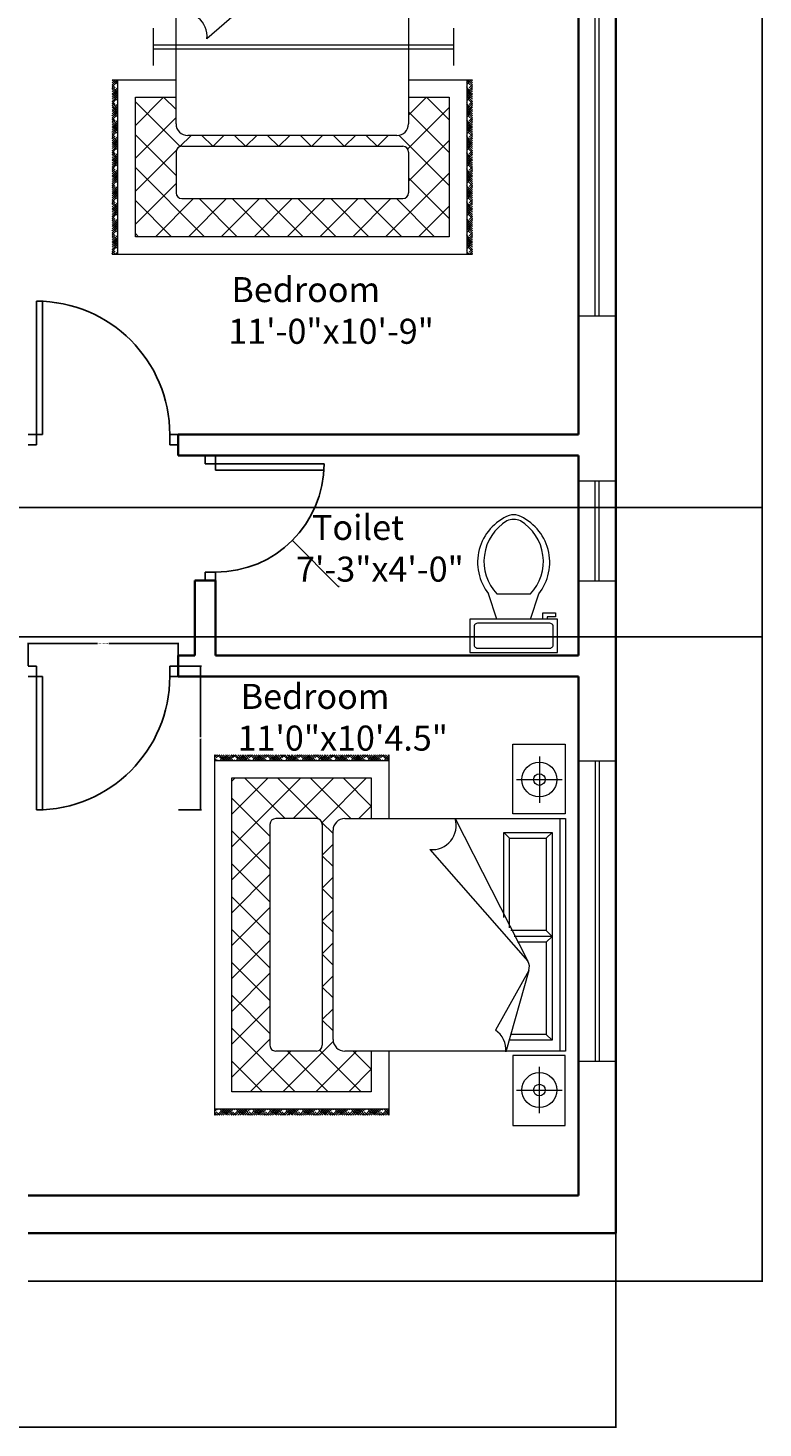
# Model space of a CAD drawing. Units: inches. Extents: x 3198 to 3702, y 1509 to 2253.
# Tile 3 of 6: x 3526 to 3702, y 1509 to 1845. Entities that reach past the tile are written whole.
import ezdxf

# ---------------------------------------------------------------- set-up
doc = ezdxf.new("R2010")
doc.units = ezdxf.units.IN
for name, color, linetype, lineweight in [('A-ANNO-DIMS', 2, 'Continuous', 18), ('A-AREA-IDEN', 7, 'Continuous', 18), ('A-DOOR', 3, 'Continuous', 25), ('A-FLOR-FIXT', 9, 'Continuous', 18), ('A-FURN', 8, 'Continuous', 13), ('A-GLAZ', 4, 'Continuous', 18), ('A-WALL', 7, 'Continuous', 35)]:
    doc.layers.add(name, color=color, linetype=linetype, lineweight=lineweight)
doc.styles.get("Standard").update_dxf_attribs({"font": 'arial.ttf'})
doc.dimstyles.get("Standard").update_dxf_attribs({"dimtxt": 0.18, "dimasz": 0.18, "dimexe": 0.18, "dimexo": 0.0625, "dimgap": 0.09, "dimtad": 0, "dimtih": 1, "dimtoh": 1, "dimdec": 4, "dimzin": 0, "dimdsep": 46, "dimtxsty": 'Standard', "dimcen": 0.09, "dimadec": 0, "dimazin": 0, "dimtfac": 1, "dimtdec": 4, "dimtofl": 0, "dimtmove": 0, "dimatfit": 3, "dimfxl": 1, "dimtolj": 1, "dimtzin": 0, "dimarcsym": 0})

# ---------------------------------------------------------------- blocks, each defined once
blk = doc.blocks.new('A$C4CB008C5')
for p, q in [((0, 3.019), (0.6, 3.019)), ((0, 2.569), (0, 3.019)), ((0.6, 3.019), (0.6, 2.569)), ((0.64, 1.121), (0.64, 3.021)), ((0.64, 3.021), (2.64, 3.021)), ((2.64, 3.021), (2.64, 1.121)), ((3.279, 3.019), (2.679, 3.019)), ((2.679, 3.019), (2.679, 2.569)), ((3.279, 2.569), (3.279, 3.019)), ((0.304, 2.6), (0.304, 2.992)), ((0.64, 2.971), (2.64, 2.971)), ((0.759, 2.905), (2.547, 2.905)), ((0.759, 2.489), (0.759, 2.905)), ((0.759, 2.905), (0.809, 2.855)), ((1.603, 2.855), (1.653, 2.905)), ((1.653, 2.905), (1.653, 2.579)), ((1.653, 2.905), (1.703, 2.855)), ((2.497, 2.855), (2.547, 2.905)), ((2.547, 2.905), (2.547, 2.54)), ((2.975, 2.6), (2.975, 2.992)), ((0.106, 2.796), (0.503, 2.796)), ((0.809, 2.855), (1.603, 2.855)), ((0.809, 2.539), (0.809, 2.855)), ((1.603, 2.855), (1.603, 2.551)), ((1.703, 2.855), (1.703, 2.607)), ((1.703, 2.855), (2.497, 2.855)), ((2.497, 2.855), (2.497, 2.556)), ((3.174, 2.796), (2.776, 2.796)), ((0.64, 2.071), (1.866, 2.698)), ((0.906, 1.854), (1.866, 2.698)), ((1.946, 2.705), (2.646, 2.507)), ((1.946, 2.705), (2.46, 2.418)), ((0.6, 2.569), (0, 2.569)), ((0.809, 2.539), (0.759, 2.489)), ((1.58, 2.539), (0.809, 2.539)), ((2.679, 2.569), (3.279, 2.569)), ((1.49, 2.489), (0.759, 2.489)), ((0.907, 1.867), (0.919, 1.867)), ((0.09, 1.5), (0.64, 1.5)), ((0.09, 1.491), (0.099, 1.5)), ((0.09, 1.473), (0.116, 1.5)), ((0.09, 1.456), (0.134, 1.5)), ((0.09, 1.474), (0.09, 1.475)), ((0.09, 1.438), (0.126, 1.474)), ((0.117, 1.43), (0.09, 1.457)), ((0.14, 1.46), (0.108, 1.492)), ((0.14, 1.478), (0.118, 1.5)), ((0.14, 1.496), (0.135, 1.5)), ((0.14, 1.442), (0.135, 1.448)), ((0.14, 0), (0.14, 1.5)), ((2.64, 1.5), (3.19, 1.5)), ((3.14, 1.496), (3.144, 1.5)), ((3.14, 1.478), (3.162, 1.5)), ((3.14, 1.5), (3.14, 0)), ((3.14, 1.46), (3.171, 1.492)), ((3.14, 1.442), (3.145, 1.448)), ((3.19, 1.456), (3.145, 1.5)), ((3.19, 1.438), (3.154, 1.474)), ((3.162, 1.43), (3.19, 1.457)), ((3.19, 1.473), (3.163, 1.5)), ((3.19, 1.491), (3.181, 1.5)), ((3.189, 1.474), (3.19, 1.475)), ((0.14, 1.389), (0.09, 1.439)), ((0.09, 1.42), (0.099, 1.43)), ((0.14, 1.372), (0.09, 1.422)), ((0.09, 1.368), (0.14, 1.417)), ((0.14, 1.354), (0.09, 1.404)), ((0.09, 1.35), (0.14, 1.4)), ((0.14, 1.336), (0.09, 1.386)), ((0.09, 1.332), (0.14, 1.382)), ((0.09, 1.314), (0.14, 1.364)), ((0.09, 1.297), (0.126, 1.333)), ((0.09, 1.333), (0.09, 1.333)), ((0.14, 1.319), (0.108, 1.35)), ((0.117, 1.412), (0.14, 1.435)), ((0.29, 1.108), (0.532, 1.35)), ((0.29, 0.15), (0.29, 1.35)), ((0.29, 1.35), (0.64, 1.35)), ((0.64, 1.243), (0.533, 1.35)), ((2.64, 1.195), (2.795, 1.35)), ((2.64, 1.35), (2.99, 1.35)), ((2.99, 1.156), (2.795, 1.35)), ((2.99, 1.35), (2.99, 0.15)), ((3.14, 1.389), (3.19, 1.439)), ((3.162, 1.412), (3.14, 1.435)), ((3.14, 1.372), (3.19, 1.422)), ((3.189, 1.368), (3.14, 1.417)), ((3.14, 1.354), (3.19, 1.404)), ((3.19, 1.35), (3.14, 1.4)), ((3.14, 1.336), (3.19, 1.386)), ((3.19, 1.332), (3.14, 1.382)), ((3.19, 1.314), (3.14, 1.364)), ((3.14, 1.319), (3.171, 1.35)), ((3.19, 1.297), (3.154, 1.333)), ((3.19, 1.42), (3.18, 1.43)), ((3.189, 1.333), (3.19, 1.333)), ((0.117, 1.288), (0.09, 1.316)), ((0.14, 1.248), (0.09, 1.298)), ((0.09, 1.279), (0.099, 1.288)), ((0.14, 1.23), (0.09, 1.28)), ((0.09, 1.227), (0.14, 1.276)), ((0.14, 1.213), (0.09, 1.263)), ((0.09, 1.208), (0.14, 1.258)), ((0.14, 1.195), (0.09, 1.245)), ((0.09, 1.19), (0.14, 1.24)), ((0.09, 1.173), (0.14, 1.223)), ((0.14, 1.177), (0.108, 1.209)), ((0.117, 1.271), (0.14, 1.294)), ((0.14, 1.301), (0.135, 1.306)), ((0.674, 0.926), (0.29, 1.31)), ((2.632, 0.904), (2.99, 1.262)), ((2.99, 0.873), (2.64, 1.223)), ((3.14, 1.301), (3.145, 1.306)), ((3.14, 1.248), (3.19, 1.298)), ((3.162, 1.271), (3.14, 1.294)), ((3.14, 1.23), (3.19, 1.28)), ((3.189, 1.227), (3.14, 1.276)), ((3.14, 1.213), (3.19, 1.263)), ((3.19, 1.208), (3.14, 1.258)), ((3.14, 1.195), (3.19, 1.245)), ((3.19, 1.19), (3.14, 1.24)), ((3.19, 1.173), (3.14, 1.223)), ((3.14, 1.177), (3.171, 1.209)), ((3.162, 1.288), (3.19, 1.316)), ((3.19, 1.279), (3.18, 1.288)), ((0.09, 1.191), (0.09, 1.192)), ((0.09, 1.155), (0.126, 1.191)), ((0.117, 1.147), (0.09, 1.174)), ((0.14, 1.107), (0.09, 1.157)), ((0.09, 1.137), (0.099, 1.147)), ((0.14, 1.089), (0.09, 1.139)), ((0.09, 1.085), (0.14, 1.134)), ((0.14, 1.071), (0.09, 1.121)), ((0.09, 1.067), (0.14, 1.117)), ((0.14, 1.054), (0.09, 1.104)), ((0.09, 1.049), (0.14, 1.099)), ((0.117, 1.129), (0.14, 1.152)), ((0.14, 1.16), (0.135, 1.165)), ((0.29, 0.825), (0.64, 1.175)), ((3.14, 1.16), (3.145, 1.165)), ((3.14, 1.107), (3.19, 1.157)), ((3.162, 1.129), (3.14, 1.152)), ((3.14, 1.089), (3.19, 1.139)), ((3.189, 1.085), (3.14, 1.134)), ((3.14, 1.071), (3.19, 1.121)), ((3.19, 1.067), (3.14, 1.117)), ((3.14, 1.054), (3.19, 1.104)), ((3.19, 1.049), (3.14, 1.099)), ((3.19, 1.155), (3.154, 1.191)), ((3.162, 1.147), (3.19, 1.174)), ((3.19, 1.137), (3.18, 1.147)), ((3.189, 1.191), (3.19, 1.192)), ((0.09, 1.031), (0.14, 1.081)), ((0.09, 1.05), (0.09, 1.051)), ((0.09, 1.014), (0.126, 1.05)), ((0.117, 1.006), (0.09, 1.033)), ((0.14, 0.965), (0.09, 1.015)), ((0.09, 0.996), (0.099, 1.006)), ((0.14, 0.948), (0.09, 0.998)), ((0.09, 0.944), (0.14, 0.993)), ((0.14, 0.93), (0.09, 0.98)), ((0.09, 0.925), (0.14, 0.975)), ((0.14, 1.036), (0.108, 1.067)), ((0.117, 0.988), (0.14, 1.011)), ((0.14, 1.018), (0.135, 1.023)), ((0.64, 0.677), (0.29, 1.027)), ((0.673, 0.925), (0.769, 1.021)), ((2.54, 1.021), (0.74, 1.021)), ((0.955, 0.928), (0.861, 1.021)), ((0.959, 0.928), (1.052, 1.021)), ((1.238, 0.928), (1.144, 1.021)), ((1.241, 0.928), (1.335, 1.021)), ((1.52, 0.928), (1.427, 1.021)), ((1.524, 0.928), (1.618, 1.021)), ((1.803, 0.928), (1.71, 1.021)), ((1.807, 0.928), (1.9, 1.021)), ((2.086, 0.928), (1.993, 1.021)), ((2.09, 0.928), (2.183, 1.021)), ((2.369, 0.928), (2.276, 1.021)), ((2.373, 0.928), (2.466, 1.021)), ((2.99, 0.59), (2.557, 1.023)), ((2.64, 0.629), (2.99, 0.979)), ((3.19, 1.031), (3.14, 1.081)), ((3.14, 1.036), (3.171, 1.067)), ((3.14, 1.018), (3.145, 1.023)), ((3.14, 0.965), (3.19, 1.015)), ((3.162, 0.988), (3.14, 1.011)), ((3.14, 0.948), (3.19, 0.998)), ((3.189, 0.944), (3.14, 0.993)), ((3.14, 0.93), (3.19, 0.98)), ((3.19, 0.925), (3.14, 0.975)), ((3.19, 1.014), (3.154, 1.05)), ((3.162, 1.006), (3.19, 1.033)), ((3.19, 0.996), (3.18, 1.006)), ((3.189, 1.05), (3.19, 1.051)), ((0.14, 0.912), (0.09, 0.962)), ((0.09, 0.908), (0.14, 0.958)), ((0.09, 0.89), (0.14, 0.94)), ((0.09, 0.908), (0.09, 0.909)), ((0.09, 0.872), (0.126, 0.908)), ((0.117, 0.864), (0.09, 0.891)), ((0.14, 0.824), (0.09, 0.874)), ((0.09, 0.855), (0.099, 0.864)), ((0.14, 0.806), (0.09, 0.856)), ((0.09, 0.802), (0.14, 0.852)), ((0.14, 0.894), (0.108, 0.926)), ((0.117, 0.847), (0.14, 0.869)), ((0.14, 0.877), (0.135, 0.882)), ((0.29, 0.542), (0.643, 0.895)), ((0.64, 0.878), (0.64, 0.528)), ((0.69, 0.928), (2.59, 0.928)), ((2.64, 0.878), (2.64, 0.528)), ((3.14, 0.912), (3.19, 0.962)), ((3.19, 0.908), (3.14, 0.958)), ((3.19, 0.89), (3.14, 0.94)), ((3.14, 0.894), (3.171, 0.926)), ((3.14, 0.877), (3.145, 0.882)), ((3.14, 0.824), (3.19, 0.874)), ((3.162, 0.847), (3.14, 0.869)), ((3.14, 0.806), (3.19, 0.856)), ((3.189, 0.802), (3.14, 0.852)), ((3.19, 0.872), (3.154, 0.908)), ((3.162, 0.864), (3.19, 0.891)), ((3.19, 0.855), (3.18, 0.864)), ((3.189, 0.908), (3.19, 0.909)), ((0.14, 0.788), (0.09, 0.838)), ((0.09, 0.784), (0.14, 0.834)), ((0.14, 0.771), (0.09, 0.821)), ((0.09, 0.766), (0.14, 0.816)), ((0.09, 0.749), (0.14, 0.799)), ((0.09, 0.767), (0.09, 0.768)), ((0.09, 0.731), (0.126, 0.767)), ((0.117, 0.723), (0.09, 0.75)), ((0.14, 0.682), (0.09, 0.732)), ((0.09, 0.713), (0.099, 0.723)), ((0.14, 0.753), (0.108, 0.785)), ((0.117, 0.705), (0.14, 0.728)), ((0.14, 0.735), (0.135, 0.74)), ((0.884, 0.15), (0.29, 0.744)), ((3.14, 0.788), (3.19, 0.838)), ((3.19, 0.784), (3.14, 0.834)), ((3.14, 0.771), (3.19, 0.821)), ((3.19, 0.766), (3.14, 0.816)), ((3.19, 0.749), (3.14, 0.799)), ((3.14, 0.753), (3.171, 0.785)), ((3.14, 0.735), (3.145, 0.74)), ((3.14, 0.682), (3.19, 0.732)), ((3.162, 0.705), (3.14, 0.728)), ((3.19, 0.731), (3.154, 0.767)), ((3.162, 0.723), (3.19, 0.75)), ((3.19, 0.713), (3.18, 0.723)), ((3.189, 0.767), (3.19, 0.768)), ((0.14, 0.665), (0.09, 0.715)), ((0.09, 0.661), (0.14, 0.71)), ((0.14, 0.647), (0.09, 0.697)), ((0.09, 0.642), (0.14, 0.692)), ((0.14, 0.629), (0.09, 0.679)), ((0.09, 0.625), (0.14, 0.675)), ((0.09, 0.607), (0.14, 0.657)), ((0.09, 0.589), (0.126, 0.626)), ((0.09, 0.626), (0.09, 0.626)), ((0.117, 0.581), (0.09, 0.609)), ((0.14, 0.612), (0.108, 0.643)), ((0.29, 0.259), (0.64, 0.609)), ((2.443, 0.15), (2.99, 0.696)), ((2.99, 0.307), (2.64, 0.657)), ((3.14, 0.665), (3.19, 0.715)), ((3.189, 0.661), (3.14, 0.71)), ((3.14, 0.647), (3.19, 0.697)), ((3.19, 0.642), (3.14, 0.692)), ((3.14, 0.629), (3.19, 0.679)), ((3.19, 0.625), (3.14, 0.675)), ((3.19, 0.607), (3.14, 0.657)), ((3.14, 0.612), (3.171, 0.643)), ((3.19, 0.589), (3.154, 0.626)), ((3.162, 0.581), (3.19, 0.609)), ((3.189, 0.626), (3.19, 0.626)), ((0.14, 0.541), (0.09, 0.591)), ((0.09, 0.572), (0.099, 0.581)), ((0.14, 0.523), (0.09, 0.573)), ((0.09, 0.519), (0.14, 0.569)), ((0.14, 0.506), (0.09, 0.556)), ((0.09, 0.501), (0.14, 0.551)), ((0.14, 0.488), (0.09, 0.538)), ((0.09, 0.483), (0.14, 0.533)), ((0.09, 0.466), (0.14, 0.516)), ((0.09, 0.484), (0.09, 0.485)), ((0.09, 0.448), (0.126, 0.484)), ((0.14, 0.47), (0.108, 0.502)), ((0.117, 0.564), (0.14, 0.586)), ((0.14, 0.594), (0.135, 0.599)), ((3.14, 0.594), (3.145, 0.599)), ((3.14, 0.541), (3.19, 0.591)), ((3.162, 0.564), (3.14, 0.586)), ((3.14, 0.523), (3.19, 0.573)), ((3.189, 0.519), (3.14, 0.569)), ((3.14, 0.506), (3.19, 0.556)), ((3.19, 0.501), (3.14, 0.551)), ((3.14, 0.488), (3.19, 0.538)), ((3.19, 0.483), (3.14, 0.533)), ((3.19, 0.466), (3.14, 0.516)), ((3.14, 0.47), (3.171, 0.502)), ((3.19, 0.448), (3.154, 0.484)), ((3.19, 0.572), (3.18, 0.581)), ((3.189, 0.484), (3.19, 0.485)), ((0.117, 0.44), (0.09, 0.467)), ((0.14, 0.399), (0.09, 0.449)), ((0.09, 0.43), (0.099, 0.44)), ((0.14, 0.382), (0.09, 0.432)), ((0.09, 0.378), (0.14, 0.427)), ((0.14, 0.364), (0.09, 0.414)), ((0.09, 0.36), (0.14, 0.41)), ((0.14, 0.346), (0.09, 0.396)), ((0.09, 0.342), (0.14, 0.392)), ((0.09, 0.324), (0.14, 0.374)), ((0.117, 0.422), (0.14, 0.445)), ((0.14, 0.453), (0.135, 0.458)), ((0.601, 0.15), (0.29, 0.462)), ((0.463, 0.15), (0.791, 0.478)), ((0.69, 0.478), (2.59, 0.478)), ((0.746, 0.15), (1.074, 0.478)), ((1.167, 0.15), (0.839, 0.478)), ((1.029, 0.15), (1.357, 0.478)), ((1.45, 0.15), (1.122, 0.478)), ((1.312, 0.15), (1.64, 0.478)), ((1.733, 0.15), (1.405, 0.478)), ((1.595, 0.15), (1.923, 0.478)), ((2.016, 0.15), (1.688, 0.478)), ((1.878, 0.15), (2.206, 0.478)), ((2.298, 0.15), (1.97, 0.478)), ((2.16, 0.15), (2.488, 0.478)), ((2.581, 0.15), (2.253, 0.478)), ((2.864, 0.15), (2.536, 0.478)), ((2.726, 0.15), (2.99, 0.414)), ((3.14, 0.453), (3.145, 0.458)), ((3.14, 0.399), (3.19, 0.449)), ((3.162, 0.422), (3.14, 0.445)), ((3.14, 0.382), (3.19, 0.432)), ((3.189, 0.378), (3.14, 0.427)), ((3.14, 0.364), (3.19, 0.414)), ((3.19, 0.36), (3.14, 0.41)), ((3.14, 0.346), (3.19, 0.396)), ((3.19, 0.342), (3.14, 0.392)), ((3.19, 0.324), (3.14, 0.374)), ((3.162, 0.44), (3.19, 0.467)), ((3.19, 0.43), (3.18, 0.44)), ((0.09, 0.307), (0.126, 0.343)), ((0.09, 0.343), (0.09, 0.343)), ((0.117, 0.299), (0.09, 0.326)), ((0.14, 0.258), (0.09, 0.308)), ((0.09, 0.289), (0.099, 0.299)), ((0.14, 0.24), (0.09, 0.29)), ((0.09, 0.237), (0.14, 0.286)), ((0.14, 0.223), (0.09, 0.273)), ((0.09, 0.218), (0.14, 0.268)), ((0.14, 0.205), (0.09, 0.255)), ((0.09, 0.201), (0.14, 0.251)), ((0.14, 0.329), (0.108, 0.36)), ((0.117, 0.281), (0.14, 0.304)), ((0.14, 0.311), (0.135, 0.316)), ((3.14, 0.329), (3.171, 0.36)), ((3.14, 0.311), (3.145, 0.316)), ((3.14, 0.258), (3.19, 0.308)), ((3.162, 0.281), (3.14, 0.304)), ((3.14, 0.24), (3.19, 0.29)), ((3.189, 0.237), (3.14, 0.286)), ((3.14, 0.223), (3.19, 0.273)), ((3.19, 0.218), (3.14, 0.268)), ((3.14, 0.205), (3.19, 0.255)), ((3.19, 0.201), (3.14, 0.251)), ((3.19, 0.307), (3.154, 0.343)), ((3.162, 0.299), (3.19, 0.326)), ((3.19, 0.289), (3.18, 0.299)), ((3.189, 0.343), (3.19, 0.343)), ((0.09, 0.183), (0.14, 0.233)), ((0.09, 0.201), (0.09, 0.202)), ((0.09, 0.165), (0.126, 0.201)), ((0.117, 0.157), (0.09, 0.184)), ((0.14, 0.117), (0.09, 0.167)), ((0.09, 0.148), (0.099, 0.157)), ((0.14, 0.099), (0.09, 0.149)), ((0.09, 0.095), (0.14, 0.144)), ((0.14, 0.081), (0.09, 0.131)), ((0.09, 0.077), (0.14, 0.127)), ((0.14, 0.187), (0.108, 0.219)), ((0.117, 0.139), (0.14, 0.162)), ((0.14, 0.17), (0.135, 0.175)), ((0.318, 0.15), (0.29, 0.179)), ((2.99, 0.15), (0.29, 0.15)), ((3.19, 0.183), (3.14, 0.233)), ((3.14, 0.187), (3.171, 0.219)), ((3.14, 0.17), (3.145, 0.175)), ((3.14, 0.117), (3.19, 0.167)), ((3.162, 0.139), (3.14, 0.162)), ((3.14, 0.099), (3.19, 0.149)), ((3.189, 0.095), (3.14, 0.144)), ((3.14, 0.081), (3.19, 0.131)), ((3.19, 0.077), (3.14, 0.127)), ((3.19, 0.165), (3.154, 0.201)), ((3.162, 0.157), (3.19, 0.184)), ((3.19, 0.148), (3.18, 0.157)), ((3.189, 0.201), (3.19, 0.202)), ((0.14, 0.064), (0.09, 0.114)), ((0.09, 0.059), (0.14, 0.109)), ((0.09, 0.041), (0.14, 0.091)), ((0.09, 0.06), (0.09, 0.061)), ((0.09, 0.024), (0.126, 0.06)), ((0.117, 0.016), (0.09, 0.043)), ((0.115, 0), (0.09, 0.025)), ((0.09, 0.006), (0.099, 0.016)), ((0.097, 0), (0.09, 0.008)), ((0.14, 0.046), (0.108, 0.078)), ((0.119, 0), (0.14, 0.021)), ((0.14, 0.028), (0.135, 0.033)), ((0.137, 0), (0.14, 0.003)), ((3.14, 0.064), (3.19, 0.114)), ((3.19, 0.059), (3.14, 0.109)), ((3.19, 0.041), (3.14, 0.091)), ((3.14, 0.046), (3.171, 0.078)), ((3.14, 0.028), (3.145, 0.033)), ((3.16, 0), (3.14, 0.021)), ((3.143, 0), (3.14, 0.003)), ((3.19, 0.024), (3.154, 0.06)), ((3.162, 0.016), (3.19, 0.043)), ((3.164, 0), (3.19, 0.025)), ((3.19, 0.006), (3.18, 0.016)), ((3.182, 0), (3.19, 0.008)), ((3.189, 0.06), (3.19, 0.061)), ((0.09, 0), (3.19, 0))]:
    blk.add_line(p, q)
for centre, radius in [((0.304, 2.796), 0.15), ((2.975, 2.796), 0.15), ((0.304, 2.796), 0.05), ((2.975, 2.796), 0.05)]:
    blk.add_circle(centre, radius)
for centre, radius, start, end in [((1.915, 2.61), 0.1, 71.7215, 119.0799), ((2.626, 2.31), 0.198, 84.1725, 146.9889), ((0.7, 1.873), 0.207, 354.6422, 106.9775), ((0.74, 1.121), 0.1, 180, 270), ((2.54, 1.121), 0.1, 270, 0), ((0.69, 0.878), 0.05, 90, 180), ((2.59, 0.878), 0.05, 0, 90), ((0.69, 0.528), 0.05, 180, 270), ((2.59, 0.528), 0.05, 270, 0)]:
    blk.add_arc(centre, radius, start, end)
blk = doc.blocks.new('*U4')
for p, q in [((9.5, -6), (9.5, -2)), ((-10, -8.5), (-8, -8.5)), ((-10, -9.5), (-10, -8.5)), ((-7, -9.5), (-10, -9.5)), ((-8, -8.5), (-8, -8)), ((-7, -8), (-7, -9.5)), ((-4, -8), (-6, -14)), ((4, -8), (6, -14)), ((4, -14), (-4, -14))]:
    blk.add_line(p, q)
blk.add_lwpolyline([(10.5, -8), (10.5, 0), (-10.5, 0), (-10.5, -8)], close=True)
for points in [[(-9.5, -2), (-9.5, -6)], [(8.5, -1), (-8.5, -1)], [(-8.5, -7), (8.5, -7)]]:
    blk.add_lwpolyline(points)
for centre, radius, start, end in [((-8.62, -1.88), 0.884, 81.8699, 188.1301), ((8.62, -1.88), 0.884, 351.8699, 98.1301), ((-8.62, -6.12), 0.884, 171.8699, 278.1301), ((8.62, -6.12), 0.884, 261.8699, 8.1301), ((3.52, -21.58), 12.17, 141.4691, 247.9714), ((4.2, -21.82), 11.33, 136.3677, 238.9468), ((-3.52, -21.58), 12.17, 292.0284, 38.5307), ((-4.2, -21.82), 11.33, 301.053, 43.6321), ((0, -27.88), 4, 245.7318, 294.2682), ((0, -29), 4, 254.8605, 285.1395)]:
    blk.add_arc(centre, radius, start, end)
blk = doc.blocks.new('DOOR-SINGLE-32')
for p, q in [((0, 34), (32, 34)), ((32, 36), (32, 34)), ((32, 34), (34.5, 34)), ((32, 32.5), (32, 34)), ((34.5, 34), (34.5, 36)), ((0.04, 32.5), (32, 32.5)), ((32, 0), (32, 2)), ((32, 2), (34.5, 2)), ((34.5, 2), (34.5, 0))]:
    blk.add_line(p, q)
blk.add_arc((32, 34), 32, 180, 270)
blk = doc.blocks.new('DOOR-SINGLE-26')
for p, q in [((0, 30), (0, 28)), ((0, 28), (2.5, 28)), ((2.5, 28), (2.5, 30)), ((2.5, 28), (28.5, 28)), ((2.5, 28), (2.5, 26.5)), ((2.5, 26.5), (28.46, 26.5)), ((0, 0), (0, 2)), ((0, 2), (2.5, 2)), ((2.5, 2), (2.5, 0))]:
    blk.add_line(p, q)
blk.add_arc((2.5, 28), 26, 270, 0)
blk = doc.blocks.new('WIN-72-W9')
for p, q in [((0, 0), (0, 9)), ((72, 0), (72, 9)), ((72, 5), (0, 5)), ((72, 4), (0, 4))]:
    blk.add_line(p, q)
blk = doc.blocks.new('WIN-24-W9')
for p, q in [((9, 24), (0, 24)), ((4, 24), (4, 0)), ((5, 24), (5, 0)), ((9, 0), (0, 0))]:
    blk.add_line(p, q)
blk = doc.blocks.new('*D21')
at = {"layer": 'A-ANNO-DIMS', "color": 0, "lineweight": -2, "transparency": 16777216}
for p, q in [((3525.55, 1691.95), (3525.55, 1697.47)), ((3525.73, 1697.29), (3542.19, 1697.29)), ((3561.37, 1697.29), (3544.91, 1697.29)), ((3561.55, 1691.95), (3561.55, 1697.47))]:
    blk.add_line(p, q, dxfattribs=at)
at = {"layer": 'A-ANNO-DIMS', "color": 0, "transparency": 16777216}
for points in [[(3525.73, 1697.32), (3525.73, 1697.26), (3525.55, 1697.29)], [(3561.37, 1697.32), (3561.37, 1697.26), (3561.55, 1697.29)]]:
    blk.add_solid(points, dxfattribs=at)
at = {"layer": 'Defpoints', "color": 0, "transparency": 16777216}
for p in [(3525.55, 1697.29), (3525.55, 1691.89), (3561.55, 1691.89)]:
    blk.add_point(p, dxfattribs=at)
at = {"layer": 'A-ANNO-DIMS', "color": 0, "transparency": 16777216, "insert": (3543.55, 1697.29), "char_height": 0.18, "attachment_point": 5}
blk.add_mtext('\\A1;ROOM DOOR 36 TYP.', dxfattribs=at)
blk = doc.blocks.new('*D22')
at = {"layer": 'A-ANNO-DIMS', "color": 0, "lineweight": -2, "transparency": 16777216}
for p, q in [((3561.61, 1691.89), (3567.13, 1691.89)), ((3566.95, 1691.71), (3566.95, 1674.82)), ((3566.95, 1657.57), (3566.95, 1674.46)), ((3561.61, 1657.39), (3567.13, 1657.39))]:
    blk.add_line(p, q, dxfattribs=at)
at = {"layer": 'A-ANNO-DIMS', "color": 0, "transparency": 16777216}
for points in [[(3566.92, 1691.71), (3566.98, 1691.71), (3566.95, 1691.89)], [(3566.92, 1657.57), (3566.98, 1657.57), (3566.95, 1657.39)]]:
    blk.add_solid(points, dxfattribs=at)
at = {"layer": 'Defpoints', "color": 0, "transparency": 16777216}
for p in [(3561.55, 1691.89), (3566.95, 1691.89), (3561.55, 1657.39)]:
    blk.add_point(p, dxfattribs=at)
at = {"layer": 'A-ANNO-DIMS', "color": 0, "transparency": 16777216, "insert": (3566.95, 1674.64), "char_height": 0.18, "attachment_point": 5}
blk.add_mtext('\\A1;35 TYP.', dxfattribs=at)
blk = doc.blocks.new('*D43')
at = {"layer": 'A-ANNO-DIMS', "color": 0, "lineweight": -2, "transparency": 16777216}
for p, q in [((3233.05, 1555.83), (3233.05, 1509.16)), ((3666.55, 1555.83), (3666.55, 1509.16)), ((3233.23, 1509.34), (3449.4, 1509.34)), ((3666.37, 1509.34), (3450.2, 1509.34))]:
    blk.add_line(p, q, dxfattribs=at)
at = {"layer": 'A-ANNO-DIMS', "color": 0, "transparency": 16777216}
for points in [[(3233.23, 1509.37), (3233.23, 1509.31), (3233.05, 1509.34)], [(3666.37, 1509.37), (3666.37, 1509.31), (3666.55, 1509.34)]]:
    blk.add_solid(points, dxfattribs=at)
at = {"layer": 'Defpoints', "color": 0, "transparency": 16777216}
for p in [(3233.05, 1555.89), (3666.55, 1555.89), (3666.55, 1509.34)]:
    blk.add_point(p, dxfattribs=at)
at = {"layer": 'A-ANNO-DIMS', "color": 0, "transparency": 16777216, "insert": (3449.8, 1509.34), "char_height": 0.18, "attachment_point": 5}
blk.add_mtext('\\A1;433.5', dxfattribs=at)
blk = doc.blocks.new('*D44')
at = {"layer": 'A-ANNO-DIMS', "color": 0, "lineweight": -2, "transparency": 16777216}
for p, q in [((3525.61, 2217.39), (3701.78, 2217.39)), ((3701.6, 2217.21), (3701.6, 1881.07)), ((3701.6, 1544.57), (3701.6, 1880.71)), ((3525.61, 1544.39), (3701.78, 1544.39))]:
    blk.add_line(p, q, dxfattribs=at)
at = {"layer": 'A-ANNO-DIMS', "color": 0, "transparency": 16777216}
for points in [[(3701.57, 2217.21), (3701.63, 2217.21), (3701.6, 2217.39)], [(3701.57, 1544.57), (3701.63, 1544.57), (3701.6, 1544.39)]]:
    blk.add_solid(points, dxfattribs=at)
at = {"layer": 'Defpoints', "color": 0, "transparency": 16777216}
for p in [(3525.55, 2217.39), (3701.6, 2217.39), (3525.55, 1544.39)]:
    blk.add_point(p, dxfattribs=at)
at = {"layer": 'A-ANNO-DIMS', "color": 0, "transparency": 16777216, "insert": (3701.6, 1880.89), "char_height": 0.18, "attachment_point": 5}
blk.add_mtext('\\A1;673', dxfattribs=at)
blk = doc.blocks.new('*D58')
at = {"layer": 'A-ANNO-DIMS', "color": 0, "lineweight": -2, "transparency": 16777216}
for p, q in [((3383.61, 1729.89), (3701.78, 1729.89)), ((3701.6, 1729.71), (3701.6, 1714.57)), ((3701.6, 1699.07), (3701.6, 1714.21)), ((3383.61, 1698.89), (3701.78, 1698.89))]:
    blk.add_line(p, q, dxfattribs=at)
at = {"layer": 'A-ANNO-DIMS', "color": 0, "transparency": 16777216}
for points in [[(3701.57, 1729.71), (3701.63, 1729.71), (3701.6, 1729.89)], [(3701.57, 1699.07), (3701.63, 1699.07), (3701.6, 1698.89)]]:
    blk.add_solid(points, dxfattribs=at)
at = {"layer": 'Defpoints', "color": 0, "transparency": 16777216}
for p in [(3383.55, 1729.89), (3701.6, 1729.89), (3383.55, 1698.89)]:
    blk.add_point(p, dxfattribs=at)
at = {"layer": 'A-ANNO-DIMS', "color": 0, "transparency": 16777216, "insert": (3701.6, 1714.39), "char_height": 0.18, "attachment_point": 5}
blk.add_mtext('\\A1;31', dxfattribs=at)
blk = doc.blocks.new('*D62')
at = {"layer": 'A-ANNO-DIMS', "color": 0, "lineweight": -2, "transparency": 16777216}
for p, q in [((3570.46, 1740.39), (3570.64, 1740.39)), ((3570.55, 1740.3), (3570.55, 1740.48)), ((3599.96, 1710.97), (3589.06, 1721.88)), ((3600.14, 1710.97), (3599.96, 1710.97))]:
    blk.add_line(p, q, dxfattribs=at)
at = {"layer": 'A-ANNO-DIMS', "color": 0, "transparency": 16777216}
blk.add_solid([(3589.08, 1721.9), (3589.04, 1721.85), (3588.93, 1722)], dxfattribs=at)
at = {"layer": 'Defpoints', "color": 0, "transparency": 16777216}
for p in [(3570.55, 1740.39), (3588.93, 1722)]:
    blk.add_point(p, dxfattribs=at)
at = {"layer": 'A-ANNO-DIMS', "color": 0, "transparency": 16777216, "insert": (3600.64, 1710.97), "char_height": 0.18, "attachment_point": 5}
blk.add_mtext('\\A1;4X R26', dxfattribs=at)

msp = doc.modelspace()

# ---------------------------------------------------------------- linework, layer by layer
at = {"layer": 'A-WALL'}
for p, q in [((3666.5475, 2205.888), (3666.5475, 1555.888)), ((3657.5475, 1747.388), (3657.5475, 1876.388)), ((3561.5475, 1747.388), (3657.5475, 1747.388)), ((3561.5475, 1747.388), (3561.5475, 1742.388)), ((3561.5475, 1742.388), (3657.5475, 1742.388)), ((3657.5475, 1694.388), (3657.5475, 1742.388)), ((3565.5475, 1694.388), (3565.5475, 1712.388)), ((3565.5475, 1712.388), (3570.5475, 1712.388)), ((3565.5475, 1712.388), (3565.5475, 1694.388)), ((3565.5475, 1712.388), (3570.5475, 1712.388)), ((3570.5475, 1694.388), (3570.5475, 1712.388)), ((3570.5475, 1712.388), (3570.5475, 1694.388)), ((3561.5475, 1694.388), (3561.5475, 1689.388)), ((3561.5475, 1694.388), (3565.5475, 1694.388)), ((3570.5475, 1694.388), (3657.5475, 1694.388)), ((3561.5475, 1689.388), (3657.5475, 1689.388)), ((3657.5475, 1564.888), (3657.5475, 1689.388)), ((3525.5475, 1564.888), (3657.5475, 1564.888)), ((3525.5475, 1555.888), (3666.5475, 1555.888))]:
    msp.add_line(p, q, dxfattribs=at)

# ---------------------------------------------------------------- block references
at = {"layer": 'A-DOOR', "extrusion": (0, 0, -1), "zscale": -1, "rotation": 269.9999999999991}
msp.add_blockref('DOOR-SINGLE-32', (-3561.5475, 1779.3885), dxfattribs=at)
at = {"layer": 'A-DOOR'}
msp.add_blockref('DOOR-SINGLE-26', (3568.047, 1712.388), dxfattribs=at)
at = {"layer": 'A-DOOR', "rotation": 89.99999999999909}
msp.add_blockref('DOOR-SINGLE-32', (3561.5475, 1657.3875), dxfattribs=at)
at = {"layer": 'A-FLOR-FIXT', "rotation": 180}
msp.add_blockref('*U4', (3642.0095, 1695.1602), dxfattribs=at)
at = {"layer": 'A-FURN', "xscale": 27.87562936897135, "yscale": 27.87562936897135, "zscale": 27.87562936897135}
msp.add_blockref('A$C4CB008C5', (3543.2133, 1790.657), dxfattribs=at)
at = {"layer": 'A-FURN', "xscale": 27.87562936897135, "yscale": 27.87562936897135, "zscale": 27.87562936897135, "rotation": 270}
msp.add_blockref('A$C4CB008C5', (3570.2384, 1673.1355), dxfattribs=at)
at = {"layer": 'A-GLAZ'}
for name, p, rotation in [('WIN-72-W9', (3657.5475, 1847.8885), 270.0000000000002), ('WIN-72-W9', (3627.5479, 1844.888), 180), ('WIN-24-W9', (3666.5479, 1736.2963), 180), ('WIN-72-W9', (3666.5475, 1597.0458), 89.99999999999935)]:
    msp.add_blockref(name, p, dxfattribs=dict(at, rotation=rotation))

# ---------------------------------------------------------------- texts
at = {"layer": 'A-AREA-IDEN', "char_height": 2.5, "attachment_point": 1}
for s, insert in [(' {\\H2.4x;Bedroom\\P11\'-0"x10\'-9"}', (3573.56, 1785.1598)), ('     {\\H2.4x;Toilet\\P7\'-3"x4\'-0"}', (3589.8162, 1728.1234)), (' {\\H2.4x;Bedroom\\P11\'0"x10\'4.5"}', (3575.7875, 1687.6042))]:
    msp.add_mtext_dynamic_manual_height_columns(s, width=40.568847, gutter_width=12.5, heights=[0], dxfattribs=dict(at, insert=insert))

# ---------------------------------------------------------------- dimensions: what is measured, and where the dimension line sits
at = {"layer": 'A-ANNO-DIMS'}
for base, p1, p2, picture, middle in [((3701.5975, 2217.388), (3525.5475, 1544.388), (3525.5475, 2217.388), '*D44', (3701.5975, 1880.888)), ((3701.5975, 1729.888), (3383.5475, 1698.888), (3383.5475, 1729.888), '*D58', (3701.5975, 1714.388))]:
    dim = msp.add_linear_dim(base=base, p1=p1, p2=p2, angle=90, dimstyle='Standard', override={"dimdec": 0, "dimlfac": 1, "dimrnd": 0, "dimzin": 0, "dimdsep": 46, "dimlunit": 2}, dxfattribs=at)
    dim.commit()
    dim.dimension.update_dxf_attribs({"geometry": picture, "text_midpoint": middle})
dim = msp.add_radius_dim(center=(3570.5475, 1740.388), mpoint=(3588.932, 1722.003), text='4X <>', dimstyle='Standard', override={"dimdec": 0, "dimlfac": 1, "dimrnd": 0, "dimzin": 0, "dimdsep": 46, "dimlunit": 2}, dxfattribs=at)
dim.commit()
dim.dimension.update_dxf_attribs({"geometry": '*D62', "text_midpoint": (3600.6447, 1710.972), "dimtype": 164})
for base, p1, p2, angle, text, picture, middle in [((3525.5475, 1697.288), (3561.5475, 1691.888), (3525.5475, 1691.888), 180, 'ROOM DOOR <> TYP.', '*D21', (3543.5475, 1697.288)), ((3566.9474569853, 1691.8880023156), (3561.5474569852, 1657.3880023156), (3561.5474569853, 1691.8880023156), 90, '<> TYP.', '*D22', (3566.9474569853, 1674.6380023156))]:
    dim = msp.add_linear_dim(base=base, p1=p1, p2=p2, angle=angle, text=text, dimstyle='Standard', override={"dimdec": 0, "dimlfac": 1, "dimrnd": 0, "dimzin": 0, "dimdsep": 46, "dimlunit": 2}, dxfattribs=at)
    dim.commit()
    dim.dimension.update_dxf_attribs({"geometry": picture, "text_midpoint": middle})
dim = msp.add_linear_dim(base=(3666.5475, 1509.338), p1=(3233.0475, 1555.888), p2=(3666.5475, 1555.888), dimstyle='Standard', override={"dimdec": 1, "dimlfac": 1, "dimrnd": 0, "dimzin": 0, "dimdsep": 46, "dimlunit": 2}, dxfattribs=at)
dim.commit()
dim.dimension.update_dxf_attribs({"geometry": '*D43', "text_midpoint": (3449.7975, 1509.338)})

doc.saveas('drawing.dxf')
